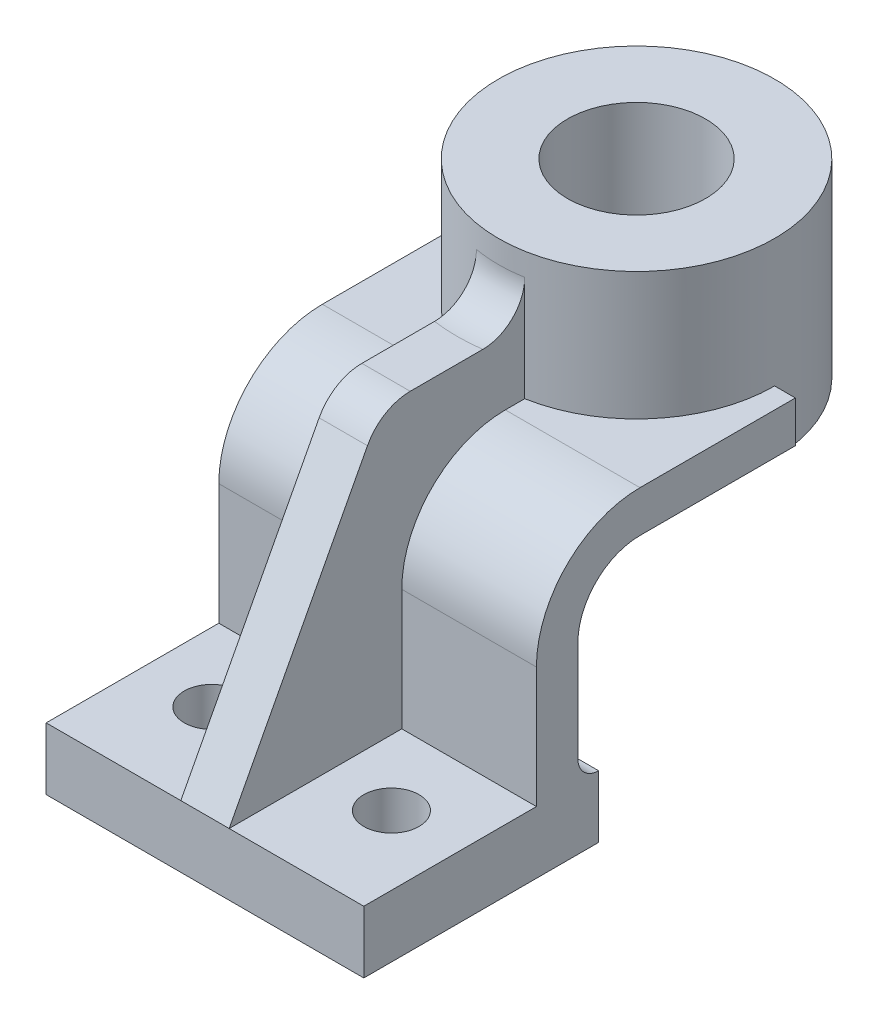
ISO-10303-21;
HEADER;
FILE_DESCRIPTION(('STEP AP214'),'2;1');
FILE_NAME('part.step','',(''),(''),'','','');
FILE_SCHEMA(('AUTOMOTIVE_DESIGN { 1 0 10303 214 1 1 1 1 }'));
ENDSEC;
DATA;
#1=APPLICATION_CONTEXT('core data for automotive mechanical design processes');
#2=APPLICATION_PROTOCOL_DEFINITION('international standard','automotive_design',2000,#1);
#3=PRODUCT_CONTEXT('',#1,'mechanical');
#4=PRODUCT('Part','Part','',(#3));
#5=PRODUCT_RELATED_PRODUCT_CATEGORY('part','',(#4));
#6=PRODUCT_DEFINITION_FORMATION('','',#4);
#7=PRODUCT_DEFINITION_CONTEXT('part definition',#1,'design');
#8=PRODUCT_DEFINITION('design','',#6,#7);
#9=PRODUCT_DEFINITION_SHAPE('','',#8);
#10=(LENGTH_UNIT() NAMED_UNIT(*) SI_UNIT(.MILLI.,.METRE.));
#11=(NAMED_UNIT(*) PLANE_ANGLE_UNIT() SI_UNIT($,.RADIAN.));
#12=(NAMED_UNIT(*) SI_UNIT($,.STERADIAN.) SOLID_ANGLE_UNIT());
#13=UNCERTAINTY_MEASURE_WITH_UNIT(LENGTH_MEASURE(1.E-05),#10,'distance_accuracy_value','');
#14=(GEOMETRIC_REPRESENTATION_CONTEXT(3) GLOBAL_UNCERTAINTY_ASSIGNED_CONTEXT((#13)) GLOBAL_UNIT_ASSIGNED_CONTEXT((#10,
#11,#12)) REPRESENTATION_CONTEXT('',''));
#15=CARTESIAN_POINT('',(0.,0.,0.));
#16=DIRECTION('',(0.,0.,1.));
#17=DIRECTION('',(1.,0.,0.));
#18=AXIS2_PLACEMENT_3D('',#15,#16,#17);
#19=CARTESIAN_POINT('',(0.,18.,0.));
#20=DIRECTION('',(0.,-1.,0.));
#21=DIRECTION('',(0.,0.,-1.));
#22=AXIS2_PLACEMENT_3D('',#19,#20,#21);
#23=PLANE('',#22);
#24=CARTESIAN_POINT('',(-26.,18.,6.));
#25=DIRECTION('',(0.,1.,0.));
#26=DIRECTION('',(0.,0.,1.));
#27=AXIS2_PLACEMENT_3D('',#24,#25,#26);
#28=CIRCLE('',#27,8.);
#29=CARTESIAN_POINT('',(-26.,18.,14.));
#30=VERTEX_POINT('',#29);
#31=EDGE_CURVE('E267',#30,#30,#28,.T.);
#32=ORIENTED_EDGE('',*,*,#31,.F.);
#33=EDGE_LOOP('',(#32));
#34=FACE_BOUND('',#33,.T.);
#35=DIRECTION('',(0.,0.,1.));
#36=VECTOR('',#35,1.);
#37=CARTESIAN_POINT('',(-7.,18.,0.));
#38=LINE('',#37,#36);
#39=CARTESIAN_POINT('',(-7.,18.,-16.));
#40=VERTEX_POINT('',#39);
#41=CARTESIAN_POINT('',(-7.,18.,34.));
#42=VERTEX_POINT('',#41);
#43=EDGE_CURVE('E228',#40,#42,#38,.T.);
#44=ORIENTED_EDGE('',*,*,#43,.F.);
#45=DIRECTION('',(1.,0.,0.));
#46=VECTOR('',#45,1.);
#47=CARTESIAN_POINT('',(-46.,18.,-16.));
#48=LINE('',#47,#46);
#49=CARTESIAN_POINT('',(-46.,18.,-16.));
#50=VERTEX_POINT('',#49);
#51=EDGE_CURVE('E266',#50,#40,#48,.T.);
#52=ORIENTED_EDGE('',*,*,#51,.F.);
#53=DIRECTION('',(0.,0.,1.));
#54=VECTOR('',#53,1.);
#55=CARTESIAN_POINT('',(-46.,18.,-34.));
#56=LINE('',#55,#54);
#57=CARTESIAN_POINT('',(-46.,18.,34.));
#58=VERTEX_POINT('',#57);
#59=EDGE_CURVE('E246',#50,#58,#56,.T.);
#60=ORIENTED_EDGE('',*,*,#59,.T.);
#61=DIRECTION('',(1.,0.,0.));
#62=VECTOR('',#61,1.);
#63=CARTESIAN_POINT('',(-46.,18.,34.));
#64=LINE('',#63,#62);
#65=EDGE_CURVE('E241',#58,#42,#64,.T.);
#66=ORIENTED_EDGE('',*,*,#65,.T.);
#67=EDGE_LOOP('',(#44,#52,#60,#66));
#68=FACE_BOUND('',#67,.T.);
#69=ADVANCED_FACE('F39',(#34,#68),#23,.F.);
#70=CARTESIAN_POINT('',(-46.,18.,-16.));
#71=DIRECTION('',(0.,0.,1.));
#72=DIRECTION('',(1.,0.,0.));
#73=AXIS2_PLACEMENT_3D('',#70,#71,#72);
#74=PLANE('',#73);
#75=ORIENTED_EDGE('',*,*,#51,.T.);
#76=DIRECTION('',(0.,1.,0.));
#77=VECTOR('',#76,1.);
#78=CARTESIAN_POINT('',(-7.,18.,-16.));
#79=LINE('',#78,#77);
#80=CARTESIAN_POINT('',(-7.,52.9999999999998,-16.));
#81=VERTEX_POINT('',#80);
#82=EDGE_CURVE('E230',#40,#81,#79,.T.);
#83=ORIENTED_EDGE('',*,*,#82,.T.);
#84=DIRECTION('',(1.,0.,0.));
#85=VECTOR('',#84,1.);
#86=CARTESIAN_POINT('',(-46.,52.9999999999998,-16.));
#87=LINE('',#86,#85);
#88=CARTESIAN_POINT('',(-46.,52.9999999999998,-16.));
#89=VERTEX_POINT('',#88);
#90=EDGE_CURVE('E298',#89,#81,#87,.T.);
#91=ORIENTED_EDGE('',*,*,#90,.F.);
#92=DIRECTION('',(0.,-1.,0.));
#93=VECTOR('',#92,1.);
#94=CARTESIAN_POINT('',(-46.,18.,-16.));
#95=LINE('',#94,#93);
#96=EDGE_CURVE('E276',#89,#50,#95,.T.);
#97=ORIENTED_EDGE('',*,*,#96,.T.);
#98=EDGE_LOOP('',(#75,#83,#91,#97));
#99=FACE_BOUND('',#98,.T.);
#100=ADVANCED_FACE('F450',(#99),#74,.T.);
#101=CARTESIAN_POINT('',(-46.,53.,-46.));
#102=DIRECTION('',(1.,0.,0.));
#103=DIRECTION('',(0.,0.,-1.));
#104=AXIS2_PLACEMENT_3D('',#101,#102,#103);
#105=CYLINDRICAL_SURFACE('',#104,30.);
#106=ORIENTED_EDGE('',*,*,#90,.T.);
#107=CARTESIAN_POINT('',(-7.,53.,-46.));
#108=DIRECTION('',(1.,0.,0.));
#109=DIRECTION('',(0.,0.,-1.));
#110=AXIS2_PLACEMENT_3D('',#107,#108,#109);
#111=CIRCLE('',#110,30.);
#112=CARTESIAN_POINT('',(-7.,83.,-46.0000000000001));
#113=VERTEX_POINT('',#112);
#114=EDGE_CURVE('E382',#81,#113,#111,.F.);
#115=ORIENTED_EDGE('',*,*,#114,.T.);
#116=DIRECTION('',(1.,0.,0.));
#117=VECTOR('',#116,1.);
#118=CARTESIAN_POINT('',(-46.,83.,-46.0000000000001));
#119=LINE('',#118,#117);
#120=CARTESIAN_POINT('',(-46.,83.,-46.0000000000001));
#121=VERTEX_POINT('',#120);
#122=EDGE_CURVE('E292',#121,#113,#119,.T.);
#123=ORIENTED_EDGE('',*,*,#122,.F.);
#124=CARTESIAN_POINT('',(-46.,53.,-46.));
#125=DIRECTION('',(1.,0.,0.));
#126=DIRECTION('',(0.,0.,-1.));
#127=AXIS2_PLACEMENT_3D('',#124,#125,#126);
#128=CIRCLE('',#127,30.);
#129=EDGE_CURVE('E321',#121,#89,#128,.T.);
#130=ORIENTED_EDGE('',*,*,#129,.T.);
#131=EDGE_LOOP('',(#106,#115,#123,#130));
#132=FACE_BOUND('',#131,.T.);
#133=ADVANCED_FACE('F455',(#132),#105,.T.);
#134=CARTESIAN_POINT('',(-46.,83.,-46.0000000000001));
#135=DIRECTION('',(0.,1.,0.));
#136=DIRECTION('',(0.,0.,1.));
#137=AXIS2_PLACEMENT_3D('',#134,#135,#136);
#138=PLANE('',#137);
#139=ORIENTED_EDGE('',*,*,#122,.T.);
#140=DIRECTION('',(0.,0.,-1.));
#141=VECTOR('',#140,1.);
#142=CARTESIAN_POINT('',(-7.,83.,-46.0000000000001));
#143=LINE('',#142,#141);
#144=CARTESIAN_POINT('',(-7.,83.,-51.6172626649696));
#145=VERTEX_POINT('',#144);
#146=EDGE_CURVE('E377',#113,#145,#143,.T.);
#147=ORIENTED_EDGE('',*,*,#146,.T.);
#148=CARTESIAN_POINT('',(0.,83.,-91.));
#149=DIRECTION('',(0.,1.,0.));
#150=DIRECTION('',(0.,0.,1.));
#151=AXIS2_PLACEMENT_3D('',#148,#149,#150);
#152=CIRCLE('',#151,40.);
#153=CARTESIAN_POINT('',(-40.,83.,-91.));
#154=VERTEX_POINT('',#153);
#155=EDGE_CURVE('E325',#154,#145,#152,.T.);
#156=ORIENTED_EDGE('',*,*,#155,.F.);
#157=DIRECTION('',(1.,0.,0.));
#158=VECTOR('',#157,1.);
#159=CARTESIAN_POINT('',(-46.,83.,-91.));
#160=LINE('',#159,#158);
#161=CARTESIAN_POINT('',(-46.,83.,-91.));
#162=VERTEX_POINT('',#161);
#163=EDGE_CURVE('E290',#162,#154,#160,.T.);
#164=ORIENTED_EDGE('',*,*,#163,.F.);
#165=DIRECTION('',(0.,0.,1.));
#166=VECTOR('',#165,1.);
#167=CARTESIAN_POINT('',(-46.,83.,-46.0000000000001));
#168=LINE('',#167,#166);
#169=EDGE_CURVE('E326',#162,#121,#168,.T.);
#170=ORIENTED_EDGE('',*,*,#169,.T.);
#171=EDGE_LOOP('',(#139,#147,#156,#164,#170));
#172=FACE_BOUND('',#171,.T.);
#173=ADVANCED_FACE('F456',(#172),#138,.T.);
#174=CARTESIAN_POINT('',(-46.,83.,-91.));
#175=DIRECTION('',(0.,0.,-1.));
#176=DIRECTION('',(-1.,0.,0.));
#177=AXIS2_PLACEMENT_3D('',#174,#175,#176);
#178=PLANE('',#177);
#179=DIRECTION('',(0.,1.,0.));
#180=VECTOR('',#179,1.);
#181=CARTESIAN_POINT('',(-40.,65.,-91.));
#182=LINE('',#181,#180);
#183=CARTESIAN_POINT('',(-40.,71.,-91.));
#184=VERTEX_POINT('',#183);
#185=EDGE_CURVE('E345',#184,#154,#182,.T.);
#186=ORIENTED_EDGE('',*,*,#185,.F.);
#187=DIRECTION('',(1.,0.,0.));
#188=VECTOR('',#187,1.);
#189=CARTESIAN_POINT('',(-46.,71.,-91.));
#190=LINE('',#189,#188);
#191=CARTESIAN_POINT('',(-46.,71.,-91.));
#192=VERTEX_POINT('',#191);
#193=EDGE_CURVE('E281',#192,#184,#190,.T.);
#194=ORIENTED_EDGE('',*,*,#193,.F.);
#195=DIRECTION('',(0.,1.,0.));
#196=VECTOR('',#195,1.);
#197=CARTESIAN_POINT('',(-46.,83.,-91.));
#198=LINE('',#197,#196);
#199=EDGE_CURVE('E327',#192,#162,#198,.T.);
#200=ORIENTED_EDGE('',*,*,#199,.T.);
#201=ORIENTED_EDGE('',*,*,#163,.T.);
#202=EDGE_LOOP('',(#186,#194,#200,#201));
#203=FACE_BOUND('',#202,.T.);
#204=ADVANCED_FACE('F462',(#203),#178,.T.);
#205=CARTESIAN_POINT('',(26.,18.,6.));
#206=DIRECTION('',(0.,1.,0.));
#207=DIRECTION('',(0.,0.,1.));
#208=AXIS2_PLACEMENT_3D('',#205,#206,#207);
#209=CIRCLE('',#208,8.);
#210=CARTESIAN_POINT('',(26.,18.,14.));
#211=VERTEX_POINT('',#210);
#212=EDGE_CURVE('E262',#211,#211,#209,.T.);
#213=ORIENTED_EDGE('',*,*,#212,.F.);
#214=EDGE_LOOP('',(#213));
#215=FACE_BOUND('',#214,.T.);
#216=CARTESIAN_POINT('',(7.,18.,-16.));
#217=VERTEX_POINT('',#216);
#218=CARTESIAN_POINT('',(46.,18.,-16.));
#219=VERTEX_POINT('',#218);
#220=EDGE_CURVE('E299',#217,#219,#48,.T.);
#221=ORIENTED_EDGE('',*,*,#220,.F.);
#222=DIRECTION('',(0.,0.,1.));
#223=VECTOR('',#222,1.);
#224=CARTESIAN_POINT('',(7.,18.,0.));
#225=LINE('',#224,#223);
#226=CARTESIAN_POINT('',(7.,18.,34.));
#227=VERTEX_POINT('',#226);
#228=EDGE_CURVE('E374',#217,#227,#225,.T.);
#229=ORIENTED_EDGE('',*,*,#228,.T.);
#230=CARTESIAN_POINT('',(46.,18.,34.));
#231=VERTEX_POINT('',#230);
#232=EDGE_CURVE('E243',#227,#231,#64,.T.);
#233=ORIENTED_EDGE('',*,*,#232,.T.);
#234=DIRECTION('',(0.,0.,1.));
#235=VECTOR('',#234,1.);
#236=CARTESIAN_POINT('',(46.,18.,-34.));
#237=LINE('',#236,#235);
#238=EDGE_CURVE('E252',#219,#231,#237,.T.);
#239=ORIENTED_EDGE('',*,*,#238,.F.);
#240=EDGE_LOOP('',(#221,#229,#233,#239));
#241=FACE_BOUND('',#240,.T.);
#242=ADVANCED_FACE('F483',(#215,#241),#23,.F.);
#243=CARTESIAN_POINT('',(-46.,18.,-34.));
#244=DIRECTION('',(0.,0.,-1.));
#245=DIRECTION('',(-1.,0.,0.));
#246=AXIS2_PLACEMENT_3D('',#243,#244,#245);
#247=PLANE('',#246);
#248=DIRECTION('',(0.,-1.,0.));
#249=VECTOR('',#248,1.);
#250=CARTESIAN_POINT('',(46.,18.,-34.));
#251=LINE('',#250,#249);
#252=CARTESIAN_POINT('',(46.,18.,-34.));
#253=VERTEX_POINT('',#252);
#254=CARTESIAN_POINT('',(46.,0.,-34.));
#255=VERTEX_POINT('',#254);
#256=EDGE_CURVE('E247',#253,#255,#251,.T.);
#257=ORIENTED_EDGE('',*,*,#256,.T.);
#258=DIRECTION('',(1.,0.,0.));
#259=VECTOR('',#258,1.);
#260=CARTESIAN_POINT('',(-46.,0.,-34.));
#261=LINE('',#260,#259);
#262=CARTESIAN_POINT('',(-46.,0.,-34.));
#263=VERTEX_POINT('',#262);
#264=EDGE_CURVE('E273',#263,#255,#261,.T.);
#265=ORIENTED_EDGE('',*,*,#264,.F.);
#266=DIRECTION('',(0.,-1.,0.));
#267=VECTOR('',#266,1.);
#268=CARTESIAN_POINT('',(-46.,18.,-34.));
#269=LINE('',#268,#267);
#270=CARTESIAN_POINT('',(-46.,18.,-34.));
#271=VERTEX_POINT('',#270);
#272=EDGE_CURVE('E530',#271,#263,#269,.T.);
#273=ORIENTED_EDGE('',*,*,#272,.F.);
#274=DIRECTION('',(1.,0.,0.));
#275=VECTOR('',#274,1.);
#276=CARTESIAN_POINT('',(-46.,18.,-34.));
#277=LINE('',#276,#275);
#278=EDGE_CURVE('E253',#271,#253,#277,.T.);
#279=ORIENTED_EDGE('',*,*,#278,.T.);
#280=EDGE_LOOP('',(#257,#265,#273,#279));
#281=FACE_BOUND('',#280,.T.);
#282=ADVANCED_FACE('F488',(#281),#247,.T.);
#283=CARTESIAN_POINT('',(-46.,18.,-34.));
#284=DIRECTION('',(1.,0.,0.));
#285=DIRECTION('',(0.,0.,-1.));
#286=AXIS2_PLACEMENT_3D('',#283,#284,#285);
#287=PLANE('',#286);
#288=DIRECTION('',(0.,0.,1.));
#289=VECTOR('',#288,1.);
#290=CARTESIAN_POINT('',(-46.,0.,-34.));
#291=LINE('',#290,#289);
#292=CARTESIAN_POINT('',(-46.,0.,34.));
#293=VERTEX_POINT('',#292);
#294=EDGE_CURVE('E256',#263,#293,#291,.T.);
#295=ORIENTED_EDGE('',*,*,#294,.T.);
#296=DIRECTION('',(0.,-1.,0.));
#297=VECTOR('',#296,1.);
#298=CARTESIAN_POINT('',(-46.,18.,34.));
#299=LINE('',#298,#297);
#300=EDGE_CURVE('E523',#58,#293,#299,.T.);
#301=ORIENTED_EDGE('',*,*,#300,.F.);
#302=ORIENTED_EDGE('',*,*,#59,.F.);
#303=ORIENTED_EDGE('',*,*,#96,.F.);
#304=ORIENTED_EDGE('',*,*,#129,.F.);
#305=ORIENTED_EDGE('',*,*,#169,.F.);
#306=ORIENTED_EDGE('',*,*,#199,.F.);
#307=DIRECTION('',(0.,0.,-1.));
#308=VECTOR('',#307,1.);
#309=CARTESIAN_POINT('',(-46.,71.,-46.0000000000001));
#310=LINE('',#309,#308);
#311=CARTESIAN_POINT('',(-46.,71.,-46.0000000000001));
#312=VERTEX_POINT('',#311);
#313=EDGE_CURVE('E333',#312,#192,#310,.T.);
#314=ORIENTED_EDGE('',*,*,#313,.F.);
#315=CARTESIAN_POINT('',(-46.,53.,-46.));
#316=DIRECTION('',(-1.,0.,0.));
#317=DIRECTION('',(0.,0.,-1.));
#318=AXIS2_PLACEMENT_3D('',#315,#316,#317);
#319=CIRCLE('',#318,18.);
#320=CARTESIAN_POINT('',(-46.,52.9999999999999,-28.));
#321=VERTEX_POINT('',#320);
#322=EDGE_CURVE('E337',#321,#312,#319,.T.);
#323=ORIENTED_EDGE('',*,*,#322,.F.);
#324=DIRECTION('',(0.,1.,0.));
#325=VECTOR('',#324,1.);
#326=CARTESIAN_POINT('',(-46.,18.,-28.));
#327=LINE('',#326,#325);
#328=CARTESIAN_POINT('',(-46.,24.,-28.));
#329=VERTEX_POINT('',#328);
#330=EDGE_CURVE('E303',#329,#321,#327,.T.);
#331=ORIENTED_EDGE('',*,*,#330,.F.);
#332=CARTESIAN_POINT('',(-46.,24.,-34.));
#333=DIRECTION('',(1.,0.,0.));
#334=DIRECTION('',(0.,0.,-1.));
#335=AXIS2_PLACEMENT_3D('',#332,#333,#334);
#336=CIRCLE('',#335,6.);
#337=EDGE_CURVE('E542',#329,#271,#336,.T.);
#338=ORIENTED_EDGE('',*,*,#337,.T.);
#339=ORIENTED_EDGE('',*,*,#272,.T.);
#340=EDGE_LOOP('',(#295,#301,#302,#303,#304,#305,#306,#314,#323,#331,#338,#339));
#341=FACE_BOUND('',#340,.T.);
#342=ADVANCED_FACE('F495',(#341),#287,.F.);
#343=CARTESIAN_POINT('',(-46.,18.,34.));
#344=DIRECTION('',(0.,0.,-1.));
#345=DIRECTION('',(-1.,0.,0.));
#346=AXIS2_PLACEMENT_3D('',#343,#344,#345);
#347=PLANE('',#346);
#348=ORIENTED_EDGE('',*,*,#232,.F.);
#349=EDGE_CURVE('E219',#42,#227,#64,.T.);
#350=ORIENTED_EDGE('',*,*,#349,.F.);
#351=ORIENTED_EDGE('',*,*,#65,.F.);
#352=ORIENTED_EDGE('',*,*,#300,.T.);
#353=DIRECTION('',(1.,0.,0.));
#354=VECTOR('',#353,1.);
#355=CARTESIAN_POINT('',(-46.,0.,34.));
#356=LINE('',#355,#354);
#357=CARTESIAN_POINT('',(46.,0.,34.));
#358=VERTEX_POINT('',#357);
#359=EDGE_CURVE('E798',#293,#358,#356,.T.);
#360=ORIENTED_EDGE('',*,*,#359,.T.);
#361=DIRECTION('',(0.,-1.,0.));
#362=VECTOR('',#361,1.);
#363=CARTESIAN_POINT('',(46.,18.,34.));
#364=LINE('',#363,#362);
#365=EDGE_CURVE('E528',#231,#358,#364,.T.);
#366=ORIENTED_EDGE('',*,*,#365,.F.);
#367=EDGE_LOOP('',(#348,#350,#351,#352,#360,#366));
#368=FACE_BOUND('',#367,.T.);
#369=ADVANCED_FACE('F237',(#368),#347,.F.);
#370=CARTESIAN_POINT('',(46.,18.,-34.));
#371=DIRECTION('',(1.,0.,0.));
#372=DIRECTION('',(0.,0.,-1.));
#373=AXIS2_PLACEMENT_3D('',#370,#371,#372);
#374=PLANE('',#373);
#375=DIRECTION('',(0.,0.,1.));
#376=VECTOR('',#375,1.);
#377=CARTESIAN_POINT('',(46.,0.,-34.));
#378=LINE('',#377,#376);
#379=EDGE_CURVE('E804',#255,#358,#378,.T.);
#380=ORIENTED_EDGE('',*,*,#379,.F.);
#381=ORIENTED_EDGE('',*,*,#256,.F.);
#382=CARTESIAN_POINT('',(46.,24.,-34.));
#383=DIRECTION('',(1.,0.,0.));
#384=DIRECTION('',(0.,0.,-1.));
#385=AXIS2_PLACEMENT_3D('',#382,#383,#384);
#386=CIRCLE('',#385,6.);
#387=CARTESIAN_POINT('',(46.,24.,-28.));
#388=VERTEX_POINT('',#387);
#389=EDGE_CURVE('E545',#253,#388,#386,.F.);
#390=ORIENTED_EDGE('',*,*,#389,.T.);
#391=DIRECTION('',(0.,1.,0.));
#392=VECTOR('',#391,1.);
#393=CARTESIAN_POINT('',(46.,18.,-28.));
#394=LINE('',#393,#392);
#395=CARTESIAN_POINT('',(46.,52.9999999999999,-28.));
#396=VERTEX_POINT('',#395);
#397=EDGE_CURVE('E316',#388,#396,#394,.T.);
#398=ORIENTED_EDGE('',*,*,#397,.T.);
#399=CARTESIAN_POINT('',(46.,53.,-46.));
#400=DIRECTION('',(-1.,0.,0.));
#401=DIRECTION('',(0.,0.,-1.));
#402=AXIS2_PLACEMENT_3D('',#399,#400,#401);
#403=CIRCLE('',#402,18.);
#404=CARTESIAN_POINT('',(46.,71.,-46.0000000000001));
#405=VERTEX_POINT('',#404);
#406=EDGE_CURVE('E317',#396,#405,#403,.T.);
#407=ORIENTED_EDGE('',*,*,#406,.T.);
#408=DIRECTION('',(0.,0.,-1.));
#409=VECTOR('',#408,1.);
#410=CARTESIAN_POINT('',(46.,71.,-46.0000000000001));
#411=LINE('',#410,#409);
#412=CARTESIAN_POINT('',(46.,71.,-91.));
#413=VERTEX_POINT('',#412);
#414=EDGE_CURVE('E312',#405,#413,#411,.T.);
#415=ORIENTED_EDGE('',*,*,#414,.T.);
#416=DIRECTION('',(0.,1.,0.));
#417=VECTOR('',#416,1.);
#418=CARTESIAN_POINT('',(46.,83.,-91.));
#419=LINE('',#418,#417);
#420=CARTESIAN_POINT('',(46.,83.,-91.));
#421=VERTEX_POINT('',#420);
#422=EDGE_CURVE('E309',#413,#421,#419,.T.);
#423=ORIENTED_EDGE('',*,*,#422,.T.);
#424=DIRECTION('',(0.,0.,1.));
#425=VECTOR('',#424,1.);
#426=CARTESIAN_POINT('',(46.,83.,-46.0000000000001));
#427=LINE('',#426,#425);
#428=CARTESIAN_POINT('',(46.,83.,-46.0000000000001));
#429=VERTEX_POINT('',#428);
#430=EDGE_CURVE('E310',#421,#429,#427,.T.);
#431=ORIENTED_EDGE('',*,*,#430,.T.);
#432=CARTESIAN_POINT('',(46.,53.,-46.));
#433=DIRECTION('',(1.,0.,0.));
#434=DIRECTION('',(0.,0.,-1.));
#435=AXIS2_PLACEMENT_3D('',#432,#433,#434);
#436=CIRCLE('',#435,30.);
#437=CARTESIAN_POINT('',(46.,52.9999999999998,-16.));
#438=VERTEX_POINT('',#437);
#439=EDGE_CURVE('E302',#429,#438,#436,.T.);
#440=ORIENTED_EDGE('',*,*,#439,.T.);
#441=DIRECTION('',(0.,-1.,0.));
#442=VECTOR('',#441,1.);
#443=CARTESIAN_POINT('',(46.,18.,-16.));
#444=LINE('',#443,#442);
#445=EDGE_CURVE('E301',#438,#219,#444,.T.);
#446=ORIENTED_EDGE('',*,*,#445,.T.);
#447=ORIENTED_EDGE('',*,*,#238,.T.);
#448=ORIENTED_EDGE('',*,*,#365,.T.);
#449=EDGE_LOOP('',(#380,#381,#390,#398,#407,#415,#423,#431,#440,#446,#447,#448));
#450=FACE_BOUND('',#449,.T.);
#451=ADVANCED_FACE('F489',(#450),#374,.T.);
#452=CARTESIAN_POINT('',(0.,0.,0.));
#453=DIRECTION('',(0.,-1.,0.));
#454=DIRECTION('',(0.,0.,-1.));
#455=AXIS2_PLACEMENT_3D('',#452,#453,#454);
#456=PLANE('',#455);
#457=ORIENTED_EDGE('',*,*,#379,.T.);
#458=ORIENTED_EDGE('',*,*,#359,.F.);
#459=ORIENTED_EDGE('',*,*,#294,.F.);
#460=ORIENTED_EDGE('',*,*,#264,.T.);
#461=EDGE_LOOP('',(#457,#458,#459,#460));
#462=FACE_BOUND('',#461,.T.);
#463=CARTESIAN_POINT('',(26.,0.,6.));
#464=DIRECTION('',(0.,1.,0.));
#465=DIRECTION('',(0.,0.,1.));
#466=AXIS2_PLACEMENT_3D('',#463,#464,#465);
#467=CIRCLE('',#466,8.);
#468=CARTESIAN_POINT('',(26.,0.,14.));
#469=VERTEX_POINT('',#468);
#470=EDGE_CURVE('E261',#469,#469,#467,.T.);
#471=ORIENTED_EDGE('',*,*,#470,.T.);
#472=EDGE_LOOP('',(#471));
#473=FACE_BOUND('',#472,.T.);
#474=CARTESIAN_POINT('',(-26.,0.,6.));
#475=DIRECTION('',(0.,1.,0.));
#476=DIRECTION('',(0.,0.,1.));
#477=AXIS2_PLACEMENT_3D('',#474,#475,#476);
#478=CIRCLE('',#477,8.);
#479=CARTESIAN_POINT('',(-26.,0.,14.));
#480=VERTEX_POINT('',#479);
#481=EDGE_CURVE('E275',#480,#480,#478,.T.);
#482=ORIENTED_EDGE('',*,*,#481,.T.);
#483=EDGE_LOOP('',(#482));
#484=FACE_BOUND('',#483,.T.);
#485=ADVANCED_FACE('F481',(#462,#473,#484),#456,.T.);
#486=CARTESIAN_POINT('',(26.,0.,6.));
#487=DIRECTION('',(0.,1.,0.));
#488=DIRECTION('',(0.,0.,1.));
#489=AXIS2_PLACEMENT_3D('',#486,#487,#488);
#490=CYLINDRICAL_SURFACE('',#489,8.);
#491=ORIENTED_EDGE('',*,*,#470,.F.);
#492=EDGE_LOOP('',(#491));
#493=FACE_BOUND('',#492,.T.);
#494=ORIENTED_EDGE('',*,*,#212,.T.);
#495=EDGE_LOOP('',(#494));
#496=FACE_BOUND('',#495,.T.);
#497=ADVANCED_FACE('F476',(#493,#496),#490,.F.);
#498=CARTESIAN_POINT('',(-26.,0.,6.));
#499=DIRECTION('',(0.,1.,0.));
#500=DIRECTION('',(0.,0.,1.));
#501=AXIS2_PLACEMENT_3D('',#498,#499,#500);
#502=CYLINDRICAL_SURFACE('',#501,8.);
#503=ORIENTED_EDGE('',*,*,#481,.F.);
#504=EDGE_LOOP('',(#503));
#505=FACE_BOUND('',#504,.T.);
#506=ORIENTED_EDGE('',*,*,#31,.T.);
#507=EDGE_LOOP('',(#506));
#508=FACE_BOUND('',#507,.T.);
#509=ADVANCED_FACE('F444',(#505,#508),#502,.F.);
#510=DIRECTION('',(0.,1.,0.));
#511=VECTOR('',#510,1.);
#512=CARTESIAN_POINT('',(7.,18.,-16.));
#513=LINE('',#512,#511);
#514=CARTESIAN_POINT('',(7.,52.9999999999998,-16.));
#515=VERTEX_POINT('',#514);
#516=EDGE_CURVE('E373',#217,#515,#513,.T.);
#517=ORIENTED_EDGE('',*,*,#516,.F.);
#518=ORIENTED_EDGE('',*,*,#220,.T.);
#519=ORIENTED_EDGE('',*,*,#445,.F.);
#520=EDGE_CURVE('E294',#515,#438,#87,.T.);
#521=ORIENTED_EDGE('',*,*,#520,.F.);
#522=EDGE_LOOP('',(#517,#518,#519,#521));
#523=FACE_BOUND('',#522,.T.);
#524=ADVANCED_FACE('F441',(#523),#74,.T.);
#525=CARTESIAN_POINT('',(7.,53.,-46.));
#526=DIRECTION('',(1.,0.,0.));
#527=DIRECTION('',(0.,0.,-1.));
#528=AXIS2_PLACEMENT_3D('',#525,#526,#527);
#529=CIRCLE('',#528,30.);
#530=CARTESIAN_POINT('',(7.,83.,-46.0000000000001));
#531=VERTEX_POINT('',#530);
#532=EDGE_CURVE('E371',#515,#531,#529,.F.);
#533=ORIENTED_EDGE('',*,*,#532,.F.);
#534=ORIENTED_EDGE('',*,*,#520,.T.);
#535=ORIENTED_EDGE('',*,*,#439,.F.);
#536=EDGE_CURVE('E289',#531,#429,#119,.T.);
#537=ORIENTED_EDGE('',*,*,#536,.F.);
#538=EDGE_LOOP('',(#533,#534,#535,#537));
#539=FACE_BOUND('',#538,.T.);
#540=ADVANCED_FACE('F443',(#539),#105,.T.);
#541=DIRECTION('',(0.,0.,-1.));
#542=VECTOR('',#541,1.);
#543=CARTESIAN_POINT('',(7.,83.,-46.0000000000001));
#544=LINE('',#543,#542);
#545=CARTESIAN_POINT('',(7.,83.,-51.6172626649696));
#546=VERTEX_POINT('',#545);
#547=EDGE_CURVE('E367',#531,#546,#544,.T.);
#548=ORIENTED_EDGE('',*,*,#547,.F.);
#549=ORIENTED_EDGE('',*,*,#536,.T.);
#550=ORIENTED_EDGE('',*,*,#430,.F.);
#551=CARTESIAN_POINT('',(40.,83.,-91.));
#552=VERTEX_POINT('',#551);
#553=EDGE_CURVE('E282',#552,#421,#160,.T.);
#554=ORIENTED_EDGE('',*,*,#553,.F.);
#555=EDGE_CURVE('E342',#546,#552,#152,.T.);
#556=ORIENTED_EDGE('',*,*,#555,.F.);
#557=EDGE_LOOP('',(#548,#549,#550,#554,#556));
#558=FACE_BOUND('',#557,.T.);
#559=ADVANCED_FACE('F448',(#558),#138,.T.);
#560=DIRECTION('',(0.,1.,0.));
#561=VECTOR('',#560,1.);
#562=CARTESIAN_POINT('',(40.,65.,-91.));
#563=LINE('',#562,#561);
#564=CARTESIAN_POINT('',(40.,71.,-91.));
#565=VERTEX_POINT('',#564);
#566=EDGE_CURVE('E343',#552,#565,#563,.F.);
#567=ORIENTED_EDGE('',*,*,#566,.F.);
#568=ORIENTED_EDGE('',*,*,#553,.T.);
#569=ORIENTED_EDGE('',*,*,#422,.F.);
#570=EDGE_CURVE('E284',#565,#413,#190,.T.);
#571=ORIENTED_EDGE('',*,*,#570,.F.);
#572=EDGE_LOOP('',(#567,#568,#569,#571));
#573=FACE_BOUND('',#572,.T.);
#574=ADVANCED_FACE('F453',(#573),#178,.T.);
#575=CARTESIAN_POINT('',(-46.,71.,-46.0000000000001));
#576=DIRECTION('',(0.,-1.,0.));
#577=DIRECTION('',(0.,0.,-1.));
#578=AXIS2_PLACEMENT_3D('',#575,#576,#577);
#579=PLANE('',#578);
#580=ORIENTED_EDGE('',*,*,#414,.F.);
#581=DIRECTION('',(1.,0.,0.));
#582=VECTOR('',#581,1.);
#583=CARTESIAN_POINT('',(-46.,71.,-46.0000000000001));
#584=LINE('',#583,#582);
#585=EDGE_CURVE('E279',#312,#405,#584,.T.);
#586=ORIENTED_EDGE('',*,*,#585,.F.);
#587=ORIENTED_EDGE('',*,*,#313,.T.);
#588=ORIENTED_EDGE('',*,*,#193,.T.);
#589=CARTESIAN_POINT('',(0.,71.,-91.));
#590=DIRECTION('',(0.,-1.,0.));
#591=DIRECTION('',(0.,0.,-1.));
#592=AXIS2_PLACEMENT_3D('',#589,#590,#591);
#593=CIRCLE('',#592,40.);
#594=EDGE_CURVE('E536',#565,#184,#593,.T.);
#595=ORIENTED_EDGE('',*,*,#594,.F.);
#596=ORIENTED_EDGE('',*,*,#570,.T.);
#597=EDGE_LOOP('',(#580,#586,#587,#588,#595,#596));
#598=FACE_BOUND('',#597,.T.);
#599=ADVANCED_FACE('F461',(#598),#579,.T.);
#600=CARTESIAN_POINT('',(-46.,53.,-46.));
#601=DIRECTION('',(1.,0.,0.));
#602=DIRECTION('',(0.,0.,-1.));
#603=AXIS2_PLACEMENT_3D('',#600,#601,#602);
#604=CYLINDRICAL_SURFACE('',#603,18.);
#605=ORIENTED_EDGE('',*,*,#406,.F.);
#606=DIRECTION('',(1.,0.,0.));
#607=VECTOR('',#606,1.);
#608=CARTESIAN_POINT('',(-46.,52.9999999999999,-28.));
#609=LINE('',#608,#607);
#610=EDGE_CURVE('E277',#321,#396,#609,.T.);
#611=ORIENTED_EDGE('',*,*,#610,.F.);
#612=ORIENTED_EDGE('',*,*,#322,.T.);
#613=ORIENTED_EDGE('',*,*,#585,.T.);
#614=EDGE_LOOP('',(#605,#611,#612,#613));
#615=FACE_BOUND('',#614,.T.);
#616=ADVANCED_FACE('F470',(#615),#604,.F.);
#617=CARTESIAN_POINT('',(-46.,18.,-28.));
#618=DIRECTION('',(0.,0.,-1.));
#619=DIRECTION('',(-1.,0.,0.));
#620=AXIS2_PLACEMENT_3D('',#617,#618,#619);
#621=PLANE('',#620);
#622=DIRECTION('',(1.,0.,0.));
#623=VECTOR('',#622,1.);
#624=CARTESIAN_POINT('',(-46.,24.,-28.));
#625=LINE('',#624,#623);
#626=EDGE_CURVE('E544',#388,#329,#625,.F.);
#627=ORIENTED_EDGE('',*,*,#626,.T.);
#628=ORIENTED_EDGE('',*,*,#330,.T.);
#629=ORIENTED_EDGE('',*,*,#610,.T.);
#630=ORIENTED_EDGE('',*,*,#397,.F.);
#631=EDGE_LOOP('',(#627,#628,#629,#630));
#632=FACE_BOUND('',#631,.T.);
#633=ADVANCED_FACE('F439',(#632),#621,.T.);
#634=CARTESIAN_POINT('',(0.,65.,-91.));
#635=DIRECTION('',(0.,1.,0.));
#636=DIRECTION('',(0.,0.,1.));
#637=AXIS2_PLACEMENT_3D('',#634,#635,#636);
#638=CYLINDRICAL_SURFACE('',#637,40.);
#639=DIRECTION('',(0.,1.,0.));
#640=VECTOR('',#639,1.);
#641=CARTESIAN_POINT('',(-7.,65.,-51.6172626649696));
#642=LINE('',#641,#640);
#643=CARTESIAN_POINT('',(-7.,113.455664300416,-51.6172626649696));
#644=VERTEX_POINT('',#643);
#645=EDGE_CURVE('E58',#145,#644,#642,.T.);
#646=ORIENTED_EDGE('',*,*,#645,.T.);
#647=CARTESIAN_POINT('',(0.,113.455664300416,-91.));
#648=DIRECTION('',(0.,1.,0.));
#649=DIRECTION('',(0.,0.,1.));
#650=AXIS2_PLACEMENT_3D('',#647,#648,#649);
#651=CIRCLE('',#650,40.);
#652=CARTESIAN_POINT('',(7.,113.455664300416,-51.6172626649696));
#653=VERTEX_POINT('',#652);
#654=EDGE_CURVE('E410',#644,#653,#651,.T.);
#655=ORIENTED_EDGE('',*,*,#654,.T.);
#656=DIRECTION('',(0.,1.,0.));
#657=VECTOR('',#656,1.);
#658=CARTESIAN_POINT('',(7.,65.,-51.6172626649696));
#659=LINE('',#658,#657);
#660=EDGE_CURVE('E66',#546,#653,#659,.T.);
#661=ORIENTED_EDGE('',*,*,#660,.F.);
#662=ORIENTED_EDGE('',*,*,#555,.T.);
#663=ORIENTED_EDGE('',*,*,#566,.T.);
#664=ORIENTED_EDGE('',*,*,#594,.T.);
#665=ORIENTED_EDGE('',*,*,#185,.T.);
#666=ORIENTED_EDGE('',*,*,#155,.T.);
#667=EDGE_LOOP('',(#646,#655,#661,#662,#663,#664,#665,#666));
#668=FACE_BOUND('',#667,.T.);
#669=CARTESIAN_POINT('',(0.,65.,-91.));
#670=DIRECTION('',(0.,1.,0.));
#671=DIRECTION('',(0.,0.,1.));
#672=AXIS2_PLACEMENT_3D('',#669,#670,#671);
#673=CIRCLE('',#672,40.);
#674=CARTESIAN_POINT('',(0.,65.,-51.));
#675=VERTEX_POINT('',#674);
#676=EDGE_CURVE('E357',#675,#675,#673,.T.);
#677=ORIENTED_EDGE('',*,*,#676,.T.);
#678=EDGE_LOOP('',(#677));
#679=FACE_BOUND('',#678,.T.);
#680=CARTESIAN_POINT('',(0.,120.,-91.));
#681=DIRECTION('',(0.,1.,0.));
#682=DIRECTION('',(0.,0.,1.));
#683=AXIS2_PLACEMENT_3D('',#680,#681,#682);
#684=CIRCLE('',#683,40.);
#685=CARTESIAN_POINT('',(0.,120.,-51.));
#686=VERTEX_POINT('',#685);
#687=EDGE_CURVE('E361',#686,#686,#684,.T.);
#688=ORIENTED_EDGE('',*,*,#687,.F.);
#689=EDGE_LOOP('',(#688));
#690=FACE_BOUND('',#689,.T.);
#691=ADVANCED_FACE('F436',(#668,#679,#690),#638,.T.);
#692=CARTESIAN_POINT('',(0.,65.,-91.));
#693=DIRECTION('',(0.,1.,0.));
#694=DIRECTION('',(0.,0.,1.));
#695=AXIS2_PLACEMENT_3D('',#692,#693,#694);
#696=PLANE('',#695);
#697=CARTESIAN_POINT('',(0.,65.,-91.));
#698=DIRECTION('',(0.,1.,0.));
#699=DIRECTION('',(0.,0.,1.));
#700=AXIS2_PLACEMENT_3D('',#697,#698,#699);
#701=CIRCLE('',#700,20.);
#702=CARTESIAN_POINT('',(0.,65.,-71.));
#703=VERTEX_POINT('',#702);
#704=EDGE_CURVE('E359',#703,#703,#701,.T.);
#705=ORIENTED_EDGE('',*,*,#704,.T.);
#706=EDGE_LOOP('',(#705));
#707=FACE_BOUND('',#706,.T.);
#708=ORIENTED_EDGE('',*,*,#676,.F.);
#709=EDGE_LOOP('',(#708));
#710=FACE_BOUND('',#709,.T.);
#711=ADVANCED_FACE('F435',(#707,#710),#696,.F.);
#712=CARTESIAN_POINT('',(0.,65.,-91.));
#713=DIRECTION('',(0.,1.,0.));
#714=DIRECTION('',(0.,0.,1.));
#715=AXIS2_PLACEMENT_3D('',#712,#713,#714);
#716=CYLINDRICAL_SURFACE('',#715,20.);
#717=CARTESIAN_POINT('',(0.,83.,-91.));
#718=DIRECTION('',(0.,1.,0.));
#719=DIRECTION('',(0.,0.,1.));
#720=AXIS2_PLACEMENT_3D('',#717,#718,#719);
#721=CIRCLE('',#720,20.);
#722=CARTESIAN_POINT('',(-20.,83.,-91.));
#723=VERTEX_POINT('',#722);
#724=CARTESIAN_POINT('',(20.,83.,-91.));
#725=VERTEX_POINT('',#724);
#726=EDGE_CURVE('E350',#723,#725,#721,.T.);
#727=ORIENTED_EDGE('',*,*,#726,.F.);
#728=DIRECTION('',(0.,1.,0.));
#729=VECTOR('',#728,1.);
#730=CARTESIAN_POINT('',(-20.,65.,-91.));
#731=LINE('',#730,#729);
#732=CARTESIAN_POINT('',(-20.,71.,-91.));
#733=VERTEX_POINT('',#732);
#734=EDGE_CURVE('E351',#733,#723,#731,.T.);
#735=ORIENTED_EDGE('',*,*,#734,.F.);
#736=CARTESIAN_POINT('',(0.,71.,-91.));
#737=DIRECTION('',(0.,-1.,0.));
#738=DIRECTION('',(0.,0.,-1.));
#739=AXIS2_PLACEMENT_3D('',#736,#737,#738);
#740=CIRCLE('',#739,20.);
#741=CARTESIAN_POINT('',(20.,71.,-91.));
#742=VERTEX_POINT('',#741);
#743=EDGE_CURVE('E529',#742,#733,#740,.T.);
#744=ORIENTED_EDGE('',*,*,#743,.F.);
#745=DIRECTION('',(0.,1.,0.));
#746=VECTOR('',#745,1.);
#747=CARTESIAN_POINT('',(20.,65.,-91.));
#748=LINE('',#747,#746);
#749=EDGE_CURVE('E352',#725,#742,#748,.F.);
#750=ORIENTED_EDGE('',*,*,#749,.F.);
#751=EDGE_LOOP('',(#727,#735,#744,#750));
#752=FACE_BOUND('',#751,.T.);
#753=ORIENTED_EDGE('',*,*,#704,.F.);
#754=EDGE_LOOP('',(#753));
#755=FACE_BOUND('',#754,.T.);
#756=CARTESIAN_POINT('',(0.,120.,-91.));
#757=DIRECTION('',(0.,1.,0.));
#758=DIRECTION('',(0.,0.,1.));
#759=AXIS2_PLACEMENT_3D('',#756,#757,#758);
#760=CIRCLE('',#759,20.);
#761=CARTESIAN_POINT('',(0.,120.,-71.));
#762=VERTEX_POINT('',#761);
#763=EDGE_CURVE('E366',#762,#762,#760,.T.);
#764=ORIENTED_EDGE('',*,*,#763,.T.);
#765=EDGE_LOOP('',(#764));
#766=FACE_BOUND('',#765,.T.);
#767=ADVANCED_FACE('F426',(#752,#755,#766),#716,.F.);
#768=CARTESIAN_POINT('',(0.,120.,-91.));
#769=DIRECTION('',(0.,1.,0.));
#770=DIRECTION('',(0.,0.,1.));
#771=AXIS2_PLACEMENT_3D('',#768,#769,#770);
#772=PLANE('',#771);
#773=ORIENTED_EDGE('',*,*,#687,.T.);
#774=EDGE_LOOP('',(#773));
#775=FACE_BOUND('',#774,.T.);
#776=ORIENTED_EDGE('',*,*,#763,.F.);
#777=EDGE_LOOP('',(#776));
#778=FACE_BOUND('',#777,.T.);
#779=ADVANCED_FACE('F425',(#775,#778),#772,.T.);
#780=EDGE_CURVE('E286',#733,#742,#190,.T.);
#781=ORIENTED_EDGE('',*,*,#780,.T.);
#782=ORIENTED_EDGE('',*,*,#743,.T.);
#783=EDGE_LOOP('',(#781,#782));
#784=FACE_BOUND('',#783,.T.);
#785=ADVANCED_FACE('F430',(#784),#579,.T.);
#786=ORIENTED_EDGE('',*,*,#780,.F.);
#787=ORIENTED_EDGE('',*,*,#734,.T.);
#788=EDGE_CURVE('E293',#723,#725,#160,.T.);
#789=ORIENTED_EDGE('',*,*,#788,.T.);
#790=ORIENTED_EDGE('',*,*,#749,.T.);
#791=EDGE_LOOP('',(#786,#787,#789,#790));
#792=FACE_BOUND('',#791,.T.);
#793=ADVANCED_FACE('F463',(#792),#178,.T.);
#794=ORIENTED_EDGE('',*,*,#788,.F.);
#795=ORIENTED_EDGE('',*,*,#726,.T.);
#796=EDGE_LOOP('',(#794,#795));
#797=FACE_BOUND('',#796,.T.);
#798=ADVANCED_FACE('F460',(#797),#138,.T.);
#799=CARTESIAN_POINT('',(0.,24.,-34.));
#800=DIRECTION('',(1.,0.,0.));
#801=DIRECTION('',(0.,0.,-1.));
#802=AXIS2_PLACEMENT_3D('',#799,#800,#801);
#803=CYLINDRICAL_SURFACE('',#802,6.);
#804=ORIENTED_EDGE('',*,*,#389,.F.);
#805=ORIENTED_EDGE('',*,*,#278,.F.);
#806=ORIENTED_EDGE('',*,*,#337,.F.);
#807=ORIENTED_EDGE('',*,*,#626,.F.);
#808=EDGE_LOOP('',(#804,#805,#806,#807));
#809=FACE_BOUND('',#808,.T.);
#810=ADVANCED_FACE('F422',(#809),#803,.F.);
#811=CARTESIAN_POINT('',(0.,101.455664300416,-52.));
#812=DIRECTION('',(0.,1.,0.));
#813=DIRECTION('',(0.,0.,1.));
#814=AXIS2_PLACEMENT_3D('',#811,#812,#813);
#815=PLANE('',#814);
#816=DIRECTION('',(0.,0.,-1.));
#817=VECTOR('',#816,1.);
#818=CARTESIAN_POINT('',(7.,101.455664300416,-48.5));
#819=LINE('',#818,#817);
#820=CARTESIAN_POINT('',(7.,101.455664300416,-39.473307888047));
#821=VERTEX_POINT('',#820);
#822=CARTESIAN_POINT('',(7.,101.455664300416,-18.4454455816237));
#823=VERTEX_POINT('',#822);
#824=EDGE_CURVE('E234',#821,#823,#819,.F.);
#825=ORIENTED_EDGE('',*,*,#824,.F.);
#826=CARTESIAN_POINT('',(0.,101.455664300416,-91.));
#827=DIRECTION('',(0.,1.,0.));
#828=DIRECTION('',(0.,0.,1.));
#829=AXIS2_PLACEMENT_3D('',#826,#827,#828);
#830=CIRCLE('',#829,52.);
#831=CARTESIAN_POINT('',(-7.,101.455664300416,-39.473307888047));
#832=VERTEX_POINT('',#831);
#833=EDGE_CURVE('E397',#821,#832,#830,.F.);
#834=ORIENTED_EDGE('',*,*,#833,.T.);
#835=DIRECTION('',(0.,0.,-1.));
#836=VECTOR('',#835,1.);
#837=CARTESIAN_POINT('',(-7.,101.455664300416,-48.5));
#838=LINE('',#837,#836);
#839=CARTESIAN_POINT('',(-7.,101.455664300416,-18.4454455816237));
#840=VERTEX_POINT('',#839);
#841=EDGE_CURVE('E223',#832,#840,#838,.F.);
#842=ORIENTED_EDGE('',*,*,#841,.T.);
#843=DIRECTION('',(1.,0.,0.));
#844=VECTOR('',#843,1.);
#845=CARTESIAN_POINT('',(0.,101.455664300416,-18.4454455816237));
#846=LINE('',#845,#844);
#847=EDGE_CURVE('E402',#840,#823,#846,.T.);
#848=ORIENTED_EDGE('',*,*,#847,.T.);
#849=EDGE_LOOP('',(#825,#834,#842,#848));
#850=FACE_BOUND('',#849,.T.);
#851=ADVANCED_FACE('F417',(#850),#815,.T.);
#852=CARTESIAN_POINT('',(0.,101.455664300416,-9.99999999999999));
#853=DIRECTION('',(0.,0.466376851848981,0.884586136031666));
#854=DIRECTION('',(0.,-0.884586136031666,0.466376851848981));
#855=AXIS2_PLACEMENT_3D('',#852,#853,#854);
#856=PLANE('',#855);
#857=DIRECTION('',(0.,-0.884586136031666,0.466376851848981));
#858=VECTOR('',#857,1.);
#859=CARTESIAN_POINT('',(7.,101.455664300416,-9.99999999999999));
#860=LINE('',#859,#858);
#861=CARTESIAN_POINT('',(7.,93.9849402263016,-6.06123967718042));
#862=VERTEX_POINT('',#861);
#863=EDGE_CURVE('E387',#862,#227,#860,.T.);
#864=ORIENTED_EDGE('',*,*,#863,.F.);
#865=DIRECTION('',(1.,0.,0.));
#866=VECTOR('',#865,1.);
#867=CARTESIAN_POINT('',(0.,93.9849402263016,-6.06123967718042));
#868=LINE('',#867,#866);
#869=CARTESIAN_POINT('',(-7.,93.9849402263016,-6.06123967718042));
#870=VERTEX_POINT('',#869);
#871=EDGE_CURVE('E218',#862,#870,#868,.F.);
#872=ORIENTED_EDGE('',*,*,#871,.T.);
#873=DIRECTION('',(0.,-0.884586136031666,0.466376851848981));
#874=VECTOR('',#873,1.);
#875=CARTESIAN_POINT('',(-7.,101.455664300416,-9.99999999999999));
#876=LINE('',#875,#874);
#877=EDGE_CURVE('E212',#870,#42,#876,.T.);
#878=ORIENTED_EDGE('',*,*,#877,.T.);
#879=ORIENTED_EDGE('',*,*,#349,.T.);
#880=EDGE_LOOP('',(#864,#872,#878,#879));
#881=FACE_BOUND('',#880,.T.);
#882=ADVANCED_FACE('F211',(#881),#856,.T.);
#883=CARTESIAN_POINT('',(7.,60.,-48.5));
#884=DIRECTION('',(1.,0.,0.));
#885=DIRECTION('',(0.,0.,-1.));
#886=AXIS2_PLACEMENT_3D('',#883,#884,#885);
#887=PLANE('',#886);
#888=ORIENTED_EDGE('',*,*,#660,.T.);
#889=CARTESIAN_POINT('',(7.,113.455664300416,-51.6172626649696));
#890=CARTESIAN_POINT('',(7.,113.121612719413,-51.6173032512437));
#891=CARTESIAN_POINT('',(7.,112.787568857384,-51.6030969601544));
#892=CARTESIAN_POINT('',(7.,112.121907236558,-51.5464854474782));
#893=CARTESIAN_POINT('',(7.,111.790289269241,-51.5040826790437));
#894=CARTESIAN_POINT('',(7.,111.132243008874,-51.3914434388541));
#895=CARTESIAN_POINT('',(7.,110.805808742686,-51.3212418523724));
#896=CARTESIAN_POINT('',(7.,110.160022743433,-51.153573943039));
#897=CARTESIAN_POINT('',(7.,109.840670979537,-51.0561077388921));
#898=CARTESIAN_POINT('',(7.,109.211207895087,-50.8346400201154));
#899=CARTESIAN_POINT('',(7.,108.901099155503,-50.7106311714998));
#900=CARTESIAN_POINT('',(7.,108.292369131346,-50.4370516817915));
#901=CARTESIAN_POINT('',(7.,107.993747962486,-50.2874807832964));
#902=CARTESIAN_POINT('',(7.,107.410059741559,-49.9639201403556));
#903=CARTESIAN_POINT('',(7.,107.124992161771,-49.7899313476848));
#904=CARTESIAN_POINT('',(7.,106.570332574621,-49.418828860804));
#905=CARTESIAN_POINT('',(7.,106.300740592576,-49.2217151287639));
#906=CARTESIAN_POINT('',(7.,105.776798443058,-48.8041803588119));
#907=CARTESIAN_POINT('',(7.,105.522583749481,-48.5835893230941));
#908=CARTESIAN_POINT('',(7.,105.033415903659,-48.1219957372938));
#909=CARTESIAN_POINT('',(7.,104.798462920242,-47.8809930083414));
#910=CARTESIAN_POINT('',(7.,104.349336470096,-47.3802535645956));
#911=CARTESIAN_POINT('',(7.,104.135167545383,-47.1205127764295));
#912=CARTESIAN_POINT('',(7.,103.729086670645,-46.5841858768845));
#913=CARTESIAN_POINT('',(7.,103.537174601217,-46.3075998558882));
#914=CARTESIAN_POINT('',(7.,103.17439522021,-45.7356091985884));
#915=CARTESIAN_POINT('',(7.,103.003852883317,-45.4399983857547));
#916=CARTESIAN_POINT('',(7.,102.688089840942,-44.8355485658647));
#917=CARTESIAN_POINT('',(7.,102.542869604284,-44.5267093140234));
#918=CARTESIAN_POINT('',(7.,102.278786718087,-43.898083947692));
#919=CARTESIAN_POINT('',(7.,102.159914071145,-43.5783020386668));
#920=CARTESIAN_POINT('',(7.,101.949296061484,-42.9300587699843));
#921=CARTESIAN_POINT('',(7.,101.85754485479,-42.6015992967612));
#922=CARTESIAN_POINT('',(7.,101.672109842913,-41.8117293930383));
#923=CARTESIAN_POINT('',(7.,101.590970758803,-41.3472792125398));
#924=CARTESIAN_POINT('',(7.,101.509814924372,-40.6465400935378));
#925=CARTESIAN_POINT('',(7.,101.489521807658,-40.4124032955817));
#926=CARTESIAN_POINT('',(7.,101.46244668098,-39.9433019174412));
#927=CARTESIAN_POINT('',(7.,101.455667422914,-39.7083371784154));
#928=CARTESIAN_POINT('',(7.,101.455664300416,-39.473307888047));
#929=B_SPLINE_CURVE_WITH_KNOTS('',3,(#889,#890,#891,#892,#893,#894,#895,#896,#897,#898,#899,
#900,#901,#902,#903,#904,#905,#906,#907,#908,#909,#910,#911,#912,#913,#914,#915,#916,#917,#918,
#919,#920,#921,#922,#923,#924,#925,#926,#927,#928),.UNSPECIFIED.,.F.,.F.,(4,2,2,2,2,2,2,2,2,2,2,
2,2,2,2,2,2,2,2,4),(0.,1.00184144249826,2.00359573410707,3.00409686873454,4.00459364744404,
5.00536723065769,6.00615089195944,7.00689555495597,8.00764185509059,9.01620353441803,
10.024774052794,11.0335644837845,12.0423495026214,13.0649794758121,14.0876283804019,
15.1098885814075,16.1319283506393,17.5427987298998,18.2475168292171,18.9523784192929),.UNSPECIFIED.);
#930=EDGE_CURVE('E11',#653,#821,#929,.T.);
#931=ORIENTED_EDGE('',*,*,#930,.T.);
#932=ORIENTED_EDGE('',*,*,#824,.T.);
#933=CARTESIAN_POINT('',(7.,87.4556643004158,-18.4454455816237));
#934=DIRECTION('',(1.,0.,0.));
#935=DIRECTION('',(0.,0.,-1.));
#936=AXIS2_PLACEMENT_3D('',#933,#934,#935);
#937=CIRCLE('',#936,14.);
#938=EDGE_CURVE('E391',#823,#862,#937,.T.);
#939=ORIENTED_EDGE('',*,*,#938,.T.);
#940=ORIENTED_EDGE('',*,*,#863,.T.);
#941=ORIENTED_EDGE('',*,*,#228,.F.);
#942=ORIENTED_EDGE('',*,*,#516,.T.);
#943=ORIENTED_EDGE('',*,*,#532,.T.);
#944=ORIENTED_EDGE('',*,*,#547,.T.);
#945=EDGE_LOOP('',(#888,#931,#932,#939,#940,#941,#942,#943,#944));
#946=FACE_BOUND('',#945,.T.);
#947=ADVANCED_FACE('F386',(#946),#887,.T.);
#948=CARTESIAN_POINT('',(-7.,60.,-48.5));
#949=DIRECTION('',(1.,0.,0.));
#950=DIRECTION('',(0.,0.,-1.));
#951=AXIS2_PLACEMENT_3D('',#948,#949,#950);
#952=PLANE('',#951);
#953=ORIENTED_EDGE('',*,*,#877,.F.);
#954=CARTESIAN_POINT('',(-7.,87.4556643004158,-18.4454455816237));
#955=DIRECTION('',(1.,0.,0.));
#956=DIRECTION('',(0.,0.,-1.));
#957=AXIS2_PLACEMENT_3D('',#954,#955,#956);
#958=CIRCLE('',#957,14.);
#959=EDGE_CURVE('E400',#870,#840,#958,.F.);
#960=ORIENTED_EDGE('',*,*,#959,.T.);
#961=ORIENTED_EDGE('',*,*,#841,.F.);
#962=CARTESIAN_POINT('',(-7.,101.455664300416,-39.473307888047));
#963=CARTESIAN_POINT('',(-7.,101.455629314222,-39.8173305196641));
#964=CARTESIAN_POINT('',(-7.,101.470188688851,-40.161345934305));
#965=CARTESIAN_POINT('',(-7.,101.528210583067,-40.8469139458257));
#966=CARTESIAN_POINT('',(-7.,101.571671617411,-41.1884666683506));
#967=CARTESIAN_POINT('',(-7.,101.687176546158,-41.8664927041082));
#968=CARTESIAN_POINT('',(-7.,101.759203225048,-42.2029689502047));
#969=CARTESIAN_POINT('',(-7.,101.931313167991,-42.8686640746859));
#970=CARTESIAN_POINT('',(-7.,102.031396165187,-43.1978830220663));
#971=CARTESIAN_POINT('',(-7.,102.258975467984,-43.8468819551049));
#972=CARTESIAN_POINT('',(-7.,102.386484771843,-44.1666573831486));
#973=CARTESIAN_POINT('',(-7.,102.668003918145,-44.7943220020174));
#974=CARTESIAN_POINT('',(-7.,102.822013676119,-45.102211230725));
#975=CARTESIAN_POINT('',(-7.,103.155443045681,-45.7038379634401));
#976=CARTESIAN_POINT('',(-7.,103.334858082349,-45.9975780026636));
#977=CARTESIAN_POINT('',(-7.,103.717883525284,-46.5688346024141));
#978=CARTESIAN_POINT('',(-7.,103.921493756553,-46.846351280259));
#979=CARTESIAN_POINT('',(-7.,104.35109399914,-47.3826131481666));
#980=CARTESIAN_POINT('',(-7.,104.577040344588,-47.6413933152456));
#981=CARTESIAN_POINT('',(-7.,105.050079422614,-48.138851979918));
#982=CARTESIAN_POINT('',(-7.,105.297172279388,-48.3775303594346));
#983=CARTESIAN_POINT('',(-7.,105.810830447455,-48.8330291453918));
#984=CARTESIAN_POINT('',(-7.,106.077399390125,-49.0498454575523));
#985=CARTESIAN_POINT('',(-7.,106.628086095089,-49.4599023714229));
#986=CARTESIAN_POINT('',(-7.,106.912203400594,-49.6531435864109));
#987=CARTESIAN_POINT('',(-7.,107.493076174342,-50.0127569371902));
#988=CARTESIAN_POINT('',(-7.,107.789678708676,-50.1793760991433));
#989=CARTESIAN_POINT('',(-7.,108.396002457961,-50.4867288317682));
#990=CARTESIAN_POINT('',(-7.,108.705723521263,-50.6274627015717));
#991=CARTESIAN_POINT('',(-7.,109.335875238839,-50.8818472946975));
#992=CARTESIAN_POINT('',(-7.,109.656298835857,-50.9955154782663));
#993=CARTESIAN_POINT('',(-7.,110.305581146113,-51.1949383368485));
#994=CARTESIAN_POINT('',(-7.,110.634437471493,-51.2807008216598));
#995=CARTESIAN_POINT('',(-7.,111.375348242688,-51.4402246297615));
#996=CARTESIAN_POINT('',(-7.,111.789031512878,-51.5066059482629));
#997=CARTESIAN_POINT('',(-7.,112.412598627423,-51.5729891205319));
#998=CARTESIAN_POINT('',(-7.,112.620854653865,-51.5895853589735));
#999=CARTESIAN_POINT('',(-7.,113.037946677855,-51.6117214378957));
#1000=CARTESIAN_POINT('',(-7.,113.246782656193,-51.6172616403215));
#1001=CARTESIAN_POINT('',(-7.,113.455664300416,-51.6172626649696));
#1002=B_SPLINE_CURVE_WITH_KNOTS('',3,(#962,#963,#964,#965,#966,#967,#968,#969,#970,#971,#972,
#973,#974,#975,#976,#977,#978,#979,#980,#981,#982,#983,#984,#985,#986,#987,#988,#989,#990,#991,
#992,#993,#994,#995,#996,#997,#998,#999,#1000,#1001),.UNSPECIFIED.,.F.,.F.,(4,2,2,2,2,2,2,2,2,2,
2,2,2,2,2,2,2,2,2,4),(0.,1.03174980052516,2.06344658395997,3.09452254243866,4.12558869418866,
5.15714458415435,6.1886971861721,7.22006426437436,8.25142388341001,9.28080569194065,
10.3101935465803,11.3397738260555,12.3693273165148,13.3886899319617,14.4080407668708,
15.4267322195984,16.4451383316487,17.6994143789669,18.3259153166722,18.952395744061),.UNSPECIFIED.);
#1003=EDGE_CURVE('E52',#832,#644,#1002,.T.);
#1004=ORIENTED_EDGE('',*,*,#1003,.T.);
#1005=ORIENTED_EDGE('',*,*,#645,.F.);
#1006=ORIENTED_EDGE('',*,*,#146,.F.);
#1007=ORIENTED_EDGE('',*,*,#114,.F.);
#1008=ORIENTED_EDGE('',*,*,#82,.F.);
#1009=ORIENTED_EDGE('',*,*,#43,.T.);
#1010=EDGE_LOOP('',(#953,#960,#961,#1004,#1005,#1006,#1007,#1008,#1009));
#1011=FACE_BOUND('',#1010,.T.);
#1012=ADVANCED_FACE('F227',(#1011),#952,.F.);
#1013=CARTESIAN_POINT('',(0.,87.4556643004158,-18.4454455816237));
#1014=DIRECTION('',(1.,0.,0.));
#1015=DIRECTION('',(0.,0.,-1.));
#1016=AXIS2_PLACEMENT_3D('',#1013,#1014,#1015);
#1017=CYLINDRICAL_SURFACE('',#1016,14.);
#1018=ORIENTED_EDGE('',*,*,#959,.F.);
#1019=ORIENTED_EDGE('',*,*,#871,.F.);
#1020=ORIENTED_EDGE('',*,*,#938,.F.);
#1021=ORIENTED_EDGE('',*,*,#847,.F.);
#1022=EDGE_LOOP('',(#1018,#1019,#1020,#1021));
#1023=FACE_BOUND('',#1022,.T.);
#1024=ADVANCED_FACE('F393',(#1023),#1017,.T.);
#1025=CARTESIAN_POINT('',(0.,113.455664300416,-91.));
#1026=DIRECTION('',(0.,1.,0.));
#1027=DIRECTION('',(0.,0.,1.));
#1028=AXIS2_PLACEMENT_3D('',#1025,#1026,#1027);
#1029=TOROIDAL_SURFACE('',#1028,52.,12.);
#1030=ORIENTED_EDGE('',*,*,#930,.F.);
#1031=ORIENTED_EDGE('',*,*,#654,.F.);
#1032=ORIENTED_EDGE('',*,*,#1003,.F.);
#1033=ORIENTED_EDGE('',*,*,#833,.F.);
#1034=EDGE_LOOP('',(#1030,#1031,#1032,#1033));
#1035=FACE_BOUND('',#1034,.T.);
#1036=ADVANCED_FACE('F41',(#1035),#1029,.F.);
#1037=CLOSED_SHELL('',(#69,#100,#133,#173,#204,#242,#282,#342,#369,#451,#485,#497,#509,#524,
#540,#559,#574,#599,#616,#633,#691,#711,#767,#779,#785,#793,#798,#810,#851,#882,#947,#1012,
#1024,#1036));
#1038=MANIFOLD_SOLID_BREP('B2',#1037);
#1039=ADVANCED_BREP_SHAPE_REPRESENTATION('',(#18,#1038),#14);
#1040=SHAPE_DEFINITION_REPRESENTATION(#9,#1039);
ENDSEC;
END-ISO-10303-21;
